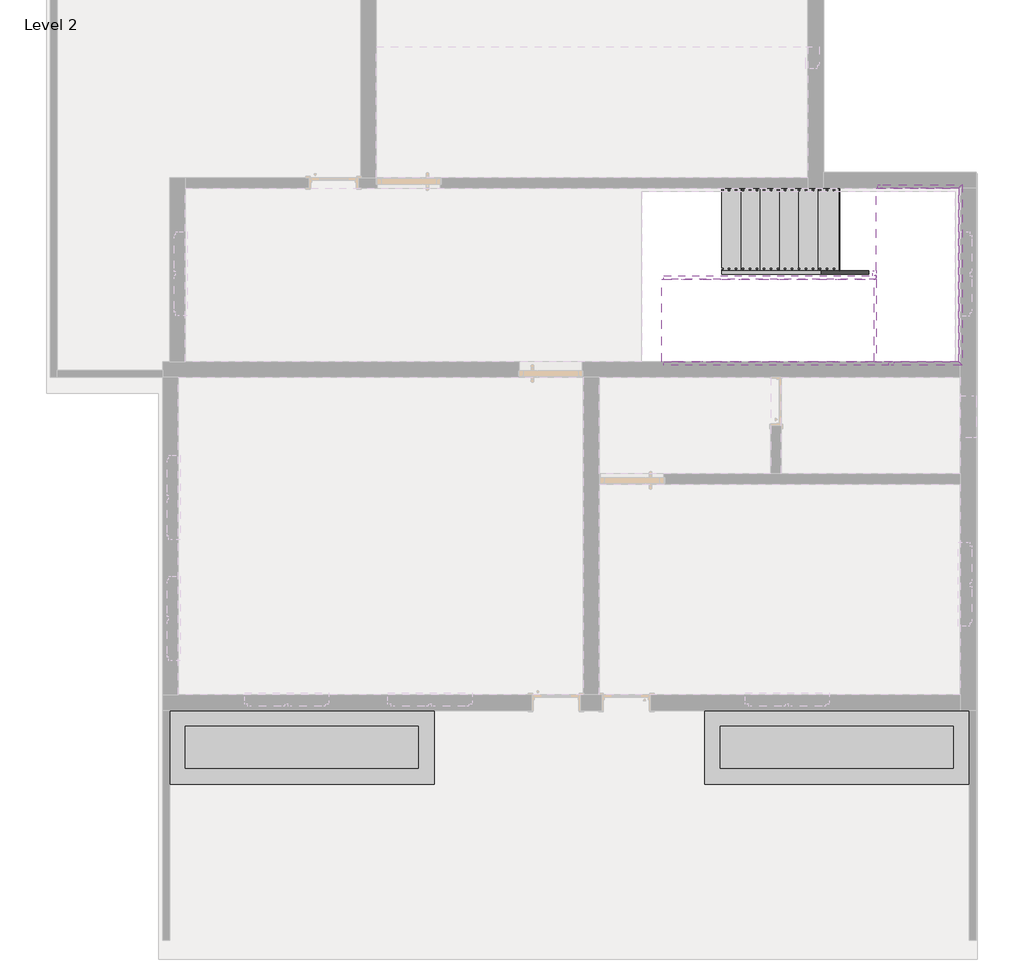
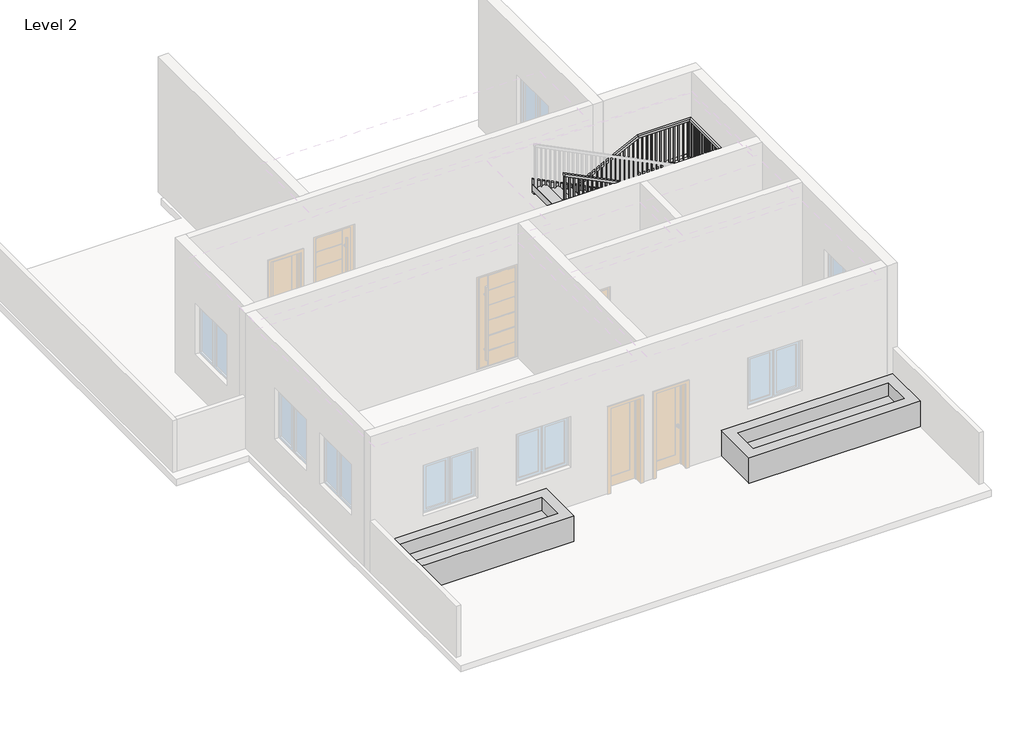
# One storey, part 3 of 3: 8 members, 2 stair flights, 1 proxy, 1 railing, 1 slab.
"""IFC4 building model written with IfcOpenShell, lengths in millimetres."""

from ifc_helpers import new_model, si_unit, frame, origin, place, context, project, spatial, polyline, outline, extrude, faceted_brep, transform, mapped, element, save
from components import generic_models_2_generic_models_2_98d2fe3e, non_monolithic_landing_0d67d91a, stair_flight_e1fa31a4, stair_flight_7751b166

model = new_model("IFC4")

# Units and contexts
model_context = context("Model", 3, world=origin())
ifc_project = project(units=[si_unit("LENGTHUNIT", "METRE", prefix="MILLI")], contexts=[model_context])

# Site, building, storey
site = spatial("IfcSite", under=ifc_project)
building = spatial("IfcBuilding", under=site)
storey = spatial("IfcBuildingStorey", under=building, Name="Level 2", Elevation=3200.4)

# Proxy
placement = place(None, origin())
generic_models_2_generic_models_2_shape = generic_models_2_generic_models_2_98d2fe3e(model_context)
element("IfcBuildingElementProxy", 1, Name="Generic Models 2 : Generic Models 2", ObjectType="Generic Models 2 : Generic Models 2", at=placement, inside=storey, context=model_context, shape_type="MappedRepresentation", body=[
    mapped(generic_models_2_generic_models_2_shape, transform((0.0, 0.0, 0.0), x_axis=(1.0, 0.0, 0.0), y_axis=(0.0, 1.0, 0.0), z_axis=(0.0, 0.0, 1.0))),
])

# Members
element("IfcMember", 2, ObjectType="Stringer - 2\" Width", at=placement, inside=storey, context=model_context, shape_type="SweptSolid", body=[
    extrude(outline(polyline([(3681.6520721, -12169.2183666), (3341.1442748, -12169.2183666), (4502.426087, -9837.43822), (4807.226087, -9909.1372097), (3681.6520721, -12169.2183666)])), frame((0.0, 3383.7503619, 0.0), z_axis=(0.0, 1.0, 0.0), x_axis=(0.0, 0.0, 1.0)), (0.0, 0.0, 1.0), 50.8),
])
element("IfcMember", 3, ObjectType="Stringer - 2\" Width", at=placement, inside=storey, context=model_context, shape_type="SweptSolid", body=[
    extrude(outline(polyline([(3681.6520721, -12169.2183666), (3341.1442748, -12169.2183666), (4429.0272787, -9984.8183666), (4769.535076, -9984.8183666), (3681.6520721, -12169.2183666)])), frame((0.0, 2139.1503619, 0.0), z_axis=(0.0, 1.0, 0.0), x_axis=(0.0, 0.0, 1.0)), (0.0, 0.0, 1.0), 50.8),
])
element("IfcMember", 4, ObjectType="Stringer - 2\" Width", at=placement, inside=storey, context=model_context, shape_type="SweptSolid", body=[
    extrude(outline(polyline([(4502.426087, -9751.1985133), (4807.226087, -9679.4995235), (6464.6085938, -13007.4183666), (6124.1007965, -13007.4183666), (4502.426087, -9751.1985133)])), frame((0.0, 818.3503619, 0.0), z_axis=(0.0, 1.0, 0.0), x_axis=(0.0, 0.0, 1.0)), (0.0, 0.0, 1.0), 50.8),
])
element("IfcMember", 5, ObjectType="Stringer - 2\" Width", at=placement, inside=storey, context=model_context, shape_type="SweptSolid", body=[
    extrude(outline(polyline([(4593.4747096, -9934.0183666), (4933.9825068, -9934.0183666), (6464.6085938, -13007.4183666), (6124.1007965, -13007.4183666), (4593.4747096, -9934.0183666)])), frame((0.0, 2062.9503619, 0.0), z_axis=(0.0, 1.0, 0.0), x_axis=(0.0, 0.0, 1.0)), (0.0, 0.0, 1.0), 50.8),
])
element("IfcMember", 6, ObjectType="Stringer - 2\" Width", at=placement, inside=storey, context=model_context, shape_type="Brep", body=[
    faceted_brep([(-9679.4995235, 869.1503619, 4807.226087), (-9679.4995235, 818.3503619, 4807.226087), (-8689.4183666, 818.3503619, 4807.226087), (-8740.2183666, 869.1503619, 4807.226087), (-9751.1985133, 869.1503619, 4502.426087), (-8740.2183666, 869.1503619, 4502.426087), (-9751.1985133, 818.3503619, 4502.426087), (-8689.4183666, 818.3503619, 4502.426087)], [[[0, 1, 2, 3]], [[4, 0, 3, 5]], [[6, 4, 5, 7]], [[1, 6, 7, 2]], [[1, 0, 4, 6]], [[2, 7, 5, 3]]]),
])
element("IfcMember", 7, ObjectType="Stringer - 2\" Width", at=placement, inside=storey, context=model_context, shape_type="SweptSolid", body=[
    extrude(outline(polyline([(-8689.4183666, 818.3503619), (-8740.2183666, 869.1503619), (-8740.2183666, 3383.7503619), (-8689.4183666, 3434.5503619), (-8689.4183666, 818.3503619)])), frame((0.0, 0.0, 4502.426087), z_axis=(0.0, 0.0, 1.0), x_axis=(1.0, 0.0, 0.0)), (0.0, 0.0, 1.0), 304.8),
])
element("IfcMember", 8, ObjectType="Stringer - 2\" Width", at=placement, inside=storey, context=model_context, shape_type="Brep", body=[
    faceted_brep([(-8740.2183666, 3383.7503619, 4807.226087), (-8689.4183666, 3434.5503619, 4807.226087), (-9909.1372097, 3434.5503619, 4807.226087), (-9909.1372097, 3383.7503619, 4807.226087), (-8740.2183666, 3383.7503619, 4502.426087), (-9837.43822, 3383.7503619, 4502.426087), (-8689.4183666, 3434.5503619, 4502.426087), (-9837.43822, 3434.5503619, 4502.426087)], [[[0, 1, 2, 3]], [[4, 0, 3, 5]], [[6, 4, 5, 7]], [[1, 6, 7, 2]], [[1, 0, 4, 6]], [[2, 7, 5, 3]]]),
])
element("IfcMember", 9, ObjectType="Stringer - 2\" Width", at=placement, inside=storey, context=model_context, shape_type="SweptSolid", body=[
    extrude(outline(polyline([(-9984.8183666, 2189.9503619), (-9934.0183666, 2189.9503619), (-9934.0183666, 2113.7503619), (-9984.8183666, 2113.7503619), (-9984.8183666, 2189.9503619)])), frame((0.0, 0.0, 4502.426087), z_axis=(0.0, 0.0, 1.0), x_axis=(1.0, 0.0, 0.0)), (0.0, 0.0, 1.0), 304.8),
])

# Railing
element("IfcRailing", 10, ObjectType="Handrail - Rectangular", at=placement, inside=storey, context=model_context, shape_type="SolidModel", body=[
    faceted_brep([(-12169.2183666, 3383.7503619, 4532.2434783), (-12169.2183666, 3383.7503619, 4475.4921787), (-12169.2183666, 3332.9503619, 4475.4921787), (-12169.2183666, 3332.9503619, 4532.2434783), (-9934.0183666, 3383.7503619, 5645.426087), (-9922.068535, 3383.7503619, 5594.626087), (-9922.068535, 3332.9503619, 5594.626087), (-9934.0183666, 3332.9503619, 5645.426087), (-8740.2183666, 3383.7503619, 5645.426087), (-8740.2183666, 3383.7503619, 5594.626087), (-8791.0183666, 3332.9503619, 5594.626087), (-8791.0183666, 3332.9503619, 5645.426087), (-8740.2183666, 869.1503619, 5645.426087), (-8740.2183666, 869.1503619, 5594.626087), (-8791.0183666, 919.9503619, 5594.626087), (-8791.0183666, 919.9503619, 5645.426087), (-9654.6183666, 869.1503619, 5645.426087), (-9666.5681983, 869.1503619, 5594.626087), (-9666.5681983, 919.9503619, 5594.626087), (-9654.6183666, 919.9503619, 5645.426087), (-9934.0183666, 869.1503619, 5784.573913), (-9956.6648951, 869.1503619, 5739.1011217), (-9956.6648951, 919.9503619, 5739.1011217), (-9934.0183666, 919.9503619, 5784.573913), (-13007.4183666, 869.1503619, 7315.2), (-13007.4183666, 919.9503619, 7315.2), (-13007.4183666, 919.9503619, 7258.4487005), (-13007.4183666, 869.1503619, 7258.4487005)], [[[0, 1, 2, 3]], [[1, 0, 4, 5]], [[2, 1, 5, 6]], [[3, 2, 6, 7]], [[0, 3, 7, 4]], [[5, 4, 8, 9]], [[6, 5, 9, 10]], [[7, 6, 10, 11]], [[4, 7, 11, 8]], [[9, 8, 12, 13]], [[10, 9, 13, 14]], [[11, 10, 14, 15]], [[8, 11, 15, 12]], [[13, 12, 16, 17]], [[14, 13, 17, 18]], [[15, 14, 18, 19]], [[12, 15, 19, 16]], [[17, 16, 20, 21]], [[18, 17, 21, 22]], [[19, 18, 22, 23]], [[16, 19, 23, 20]], [[24, 25, 26, 27]], [[21, 20, 24, 27]], [[22, 21, 27, 26]], [[23, 22, 26, 25]], [[20, 23, 25, 24]]]),
    extrude(outline(polyline([(7250.542574, -12991.5433666), (6261.6521739, -12991.5433666), (6261.6521739, -12972.4933666), (7241.0552222, -12972.4933666), (7250.542574, -12991.5433666)])), frame((0.0, 885.0253619, 0.0), z_axis=(0.0, 1.0, 0.0), x_axis=(0.0, 0.0, 1.0)), (0.0, 0.0, 1.0), 19.05),
    extrude(outline(polyline([(7199.9433645, -12889.9433666), (6261.6521739, -12889.9433666), (6261.6521739, -12870.8933666), (7190.4560127, -12870.8933666), (7199.9433645, -12889.9433666)])), frame((0.0, 885.0253619, 0.0), z_axis=(0.0, 1.0, 0.0), x_axis=(0.0, 0.0, 1.0)), (0.0, 0.0, 1.0), 19.05),
    extrude(outline(polyline([(7149.344155, -12788.3433666), (6261.6521739, -12788.3433666), (6261.6521739, -12769.2933666), (7139.8568032, -12769.2933666), (7149.344155, -12788.3433666)])), frame((0.0, 885.0253619, 0.0), z_axis=(0.0, 1.0, 0.0), x_axis=(0.0, 0.0, 1.0)), (0.0, 0.0, 1.0), 19.05),
    extrude(outline(polyline([(7098.7449455, -12686.7433666), (6122.5043478, -12686.7433666), (6122.5043478, -12667.6933666), (7089.2575937, -12667.6933666), (7098.7449455, -12686.7433666)])), frame((0.0, 885.0253619, 0.0), z_axis=(0.0, 1.0, 0.0), x_axis=(0.0, 0.0, 1.0)), (0.0, 0.0, 1.0), 19.05),
    extrude(outline(polyline([(7048.145736, -12585.1433666), (6122.5043478, -12585.1433666), (6122.5043478, -12566.0933666), (7038.6583842, -12566.0933666), (7048.145736, -12585.1433666)])), frame((0.0, 885.0253619, 0.0), z_axis=(0.0, 1.0, 0.0), x_axis=(0.0, 0.0, 1.0)), (0.0, 0.0, 1.0), 19.05),
    extrude(outline(polyline([(6997.5465265, -12483.5433666), (6122.5043478, -12483.5433666), (6122.5043478, -12464.4933666), (6988.0591748, -12464.4933666), (6997.5465265, -12483.5433666)])), frame((0.0, 885.0253619, 0.0), z_axis=(0.0, 1.0, 0.0), x_axis=(0.0, 0.0, 1.0)), (0.0, 0.0, 1.0), 19.05),
    extrude(outline(polyline([(6946.9473171, -12381.9433666), (5983.3565217, -12381.9433666), (5983.3565217, -12362.8933666), (6937.4599653, -12362.8933666), (6946.9473171, -12381.9433666)])), frame((0.0, 885.0253619, 0.0), z_axis=(0.0, 1.0, 0.0), x_axis=(0.0, 0.0, 1.0)), (0.0, 0.0, 1.0), 19.05),
    extrude(outline(polyline([(6896.3481076, -12280.3433666), (5983.3565217, -12280.3433666), (5983.3565217, -12261.2933666), (6886.8607558, -12261.2933666), (6896.3481076, -12280.3433666)])), frame((0.0, 885.0253619, 0.0), z_axis=(0.0, 1.0, 0.0), x_axis=(0.0, 0.0, 1.0)), (0.0, 0.0, 1.0), 19.05),
    extrude(outline(polyline([(6845.7488981, -12178.7433666), (5983.3565217, -12178.7433666), (5983.3565217, -12159.6933666), (6836.2615463, -12159.6933666), (6845.7488981, -12178.7433666)])), frame((0.0, 885.0253619, 0.0), z_axis=(0.0, 1.0, 0.0), x_axis=(0.0, 0.0, 1.0)), (0.0, 0.0, 1.0), 19.05),
    extrude(outline(polyline([(6795.1496886, -12077.1433666), (5844.2086957, -12077.1433666), (5844.2086957, -12058.0933666), (6785.6623368, -12058.0933666), (6795.1496886, -12077.1433666)])), frame((0.0, 885.0253619, 0.0), z_axis=(0.0, 1.0, 0.0), x_axis=(0.0, 0.0, 1.0)), (0.0, 0.0, 1.0), 19.05),
    extrude(outline(polyline([(6744.5504791, -11975.5433666), (5844.2086957, -11975.5433666), (5844.2086957, -11956.4933666), (6735.0631273, -11956.4933666), (6744.5504791, -11975.5433666)])), frame((0.0, 885.0253619, 0.0), z_axis=(0.0, 1.0, 0.0), x_axis=(0.0, 0.0, 1.0)), (0.0, 0.0, 1.0), 19.05),
    extrude(outline(polyline([(6693.9512696, -11873.9433666), (5705.0608696, -11873.9433666), (5705.0608696, -11854.8933666), (6684.4639178, -11854.8933666), (6693.9512696, -11873.9433666)])), frame((0.0, 885.0253619, 0.0), z_axis=(0.0, 1.0, 0.0), x_axis=(0.0, 0.0, 1.0)), (0.0, 0.0, 1.0), 19.05),
    extrude(outline(polyline([(6643.3520601, -11772.3433666), (5705.0608696, -11772.3433666), (5705.0608696, -11753.2933666), (6633.8647084, -11753.2933666), (6643.3520601, -11772.3433666)])), frame((0.0, 885.0253619, 0.0), z_axis=(0.0, 1.0, 0.0), x_axis=(0.0, 0.0, 1.0)), (0.0, 0.0, 1.0), 19.05),
    extrude(outline(polyline([(6592.7528507, -11670.7433666), (5705.0608696, -11670.7433666), (5705.0608696, -11651.6933666), (6583.2654989, -11651.6933666), (6592.7528507, -11670.7433666)])), frame((0.0, 885.0253619, 0.0), z_axis=(0.0, 1.0, 0.0), x_axis=(0.0, 0.0, 1.0)), (0.0, 0.0, 1.0), 19.05),
    extrude(outline(polyline([(6542.1536412, -11569.1433666), (5565.9130435, -11569.1433666), (5565.9130435, -11550.0933666), (6532.6662894, -11550.0933666), (6542.1536412, -11569.1433666)])), frame((0.0, 885.0253619, 0.0), z_axis=(0.0, 1.0, 0.0), x_axis=(0.0, 0.0, 1.0)), (0.0, 0.0, 1.0), 19.05),
    extrude(outline(polyline([(6491.5544317, -11467.5433666), (5565.9130435, -11467.5433666), (5565.9130435, -11448.4933666), (6482.0670799, -11448.4933666), (6491.5544317, -11467.5433666)])), frame((0.0, 885.0253619, 0.0), z_axis=(0.0, 1.0, 0.0), x_axis=(0.0, 0.0, 1.0)), (0.0, 0.0, 1.0), 19.05),
    extrude(outline(polyline([(6440.9552222, -11365.9433666), (5565.9130435, -11365.9433666), (5565.9130435, -11346.8933666), (6431.4678704, -11346.8933666), (6440.9552222, -11365.9433666)])), frame((0.0, 885.0253619, 0.0), z_axis=(0.0, 1.0, 0.0), x_axis=(0.0, 0.0, 1.0)), (0.0, 0.0, 1.0), 19.05),
    extrude(outline(polyline([(6390.3560127, -11264.3433666), (5426.7652174, -11264.3433666), (5426.7652174, -11245.2933666), (6380.8686609, -11245.2933666), (6390.3560127, -11264.3433666)])), frame((0.0, 885.0253619, 0.0), z_axis=(0.0, 1.0, 0.0), x_axis=(0.0, 0.0, 1.0)), (0.0, 0.0, 1.0), 19.05),
    extrude(outline(polyline([(6339.7568032, -11162.7433666), (5426.7652174, -11162.7433666), (5426.7652174, -11143.6933666), (6330.2694514, -11143.6933666), (6339.7568032, -11162.7433666)])), frame((0.0, 885.0253619, 0.0), z_axis=(0.0, 1.0, 0.0), x_axis=(0.0, 0.0, 1.0)), (0.0, 0.0, 1.0), 19.05),
    extrude(outline(polyline([(6289.1575937, -11061.1433666), (5426.7652174, -11061.1433666), (5426.7652174, -11042.0933666), (6279.670242, -11042.0933666), (6289.1575937, -11061.1433666)])), frame((0.0, 885.0253619, 0.0), z_axis=(0.0, 1.0, 0.0), x_axis=(0.0, 0.0, 1.0)), (0.0, 0.0, 1.0), 19.05),
    extrude(outline(polyline([(6238.5583842, -10959.5433666), (5287.6173913, -10959.5433666), (5287.6173913, -10940.4933666), (6229.0710325, -10940.4933666), (6238.5583842, -10959.5433666)])), frame((0.0, 885.0253619, 0.0), z_axis=(0.0, 1.0, 0.0), x_axis=(0.0, 0.0, 1.0)), (0.0, 0.0, 1.0), 19.05),
    extrude(outline(polyline([(6187.9591748, -10857.9433666), (5287.6173913, -10857.9433666), (5287.6173913, -10838.8933666), (6178.471823, -10838.8933666), (6187.9591748, -10857.9433666)])), frame((0.0, 885.0253619, 0.0), z_axis=(0.0, 1.0, 0.0), x_axis=(0.0, 0.0, 1.0)), (0.0, 0.0, 1.0), 19.05),
    extrude(outline(polyline([(6137.3599653, -10756.3433666), (5148.4695652, -10756.3433666), (5148.4695652, -10737.2933666), (6127.8726135, -10737.2933666), (6137.3599653, -10756.3433666)])), frame((0.0, 885.0253619, 0.0), z_axis=(0.0, 1.0, 0.0), x_axis=(0.0, 0.0, 1.0)), (0.0, 0.0, 1.0), 19.05),
    extrude(outline(polyline([(6086.7607558, -10654.7433666), (5148.4695652, -10654.7433666), (5148.4695652, -10635.6933666), (6077.273404, -10635.6933666), (6086.7607558, -10654.7433666)])), frame((0.0, 885.0253619, 0.0), z_axis=(0.0, 1.0, 0.0), x_axis=(0.0, 0.0, 1.0)), (0.0, 0.0, 1.0), 19.05),
    extrude(outline(polyline([(6036.1615463, -10553.1433666), (5148.4695652, -10553.1433666), (5148.4695652, -10534.0933666), (6026.6741945, -10534.0933666), (6036.1615463, -10553.1433666)])), frame((0.0, 885.0253619, 0.0), z_axis=(0.0, 1.0, 0.0), x_axis=(0.0, 0.0, 1.0)), (0.0, 0.0, 1.0), 19.05),
    extrude(outline(polyline([(5985.5623368, -10451.5433666), (5009.3217391, -10451.5433666), (5009.3217391, -10432.4933666), (5976.074985, -10432.4933666), (5985.5623368, -10451.5433666)])), frame((0.0, 885.0253619, 0.0), z_axis=(0.0, 1.0, 0.0), x_axis=(0.0, 0.0, 1.0)), (0.0, 0.0, 1.0), 19.05),
    extrude(outline(polyline([(5934.9631273, -10349.9433666), (5009.3217391, -10349.9433666), (5009.3217391, -10330.8933666), (5925.4757756, -10330.8933666), (5934.9631273, -10349.9433666)])), frame((0.0, 885.0253619, 0.0), z_axis=(0.0, 1.0, 0.0), x_axis=(0.0, 0.0, 1.0)), (0.0, 0.0, 1.0), 19.05),
    extrude(outline(polyline([(5884.3639178, -10248.3433666), (5009.3217391, -10248.3433666), (5009.3217391, -10229.2933666), (5874.8765661, -10229.2933666), (5884.3639178, -10248.3433666)])), frame((0.0, 885.0253619, 0.0), z_axis=(0.0, 1.0, 0.0), x_axis=(0.0, 0.0, 1.0)), (0.0, 0.0, 1.0), 19.05),
    extrude(outline(polyline([(5833.7647084, -10146.7433666), (4870.173913, -10146.7433666), (4870.173913, -10127.6933666), (5824.2773566, -10127.6933666), (5833.7647084, -10146.7433666)])), frame((0.0, 885.0253619, 0.0), z_axis=(0.0, 1.0, 0.0), x_axis=(0.0, 0.0, 1.0)), (0.0, 0.0, 1.0), 19.05),
    extrude(outline(polyline([(5783.1654989, -10045.1433666), (4870.173913, -10045.1433666), (4870.173913, -10026.0933666), (5773.6781471, -10026.0933666), (5783.1654989, -10045.1433666)])), frame((0.0, 885.0253619, 0.0), z_axis=(0.0, 1.0, 0.0), x_axis=(0.0, 0.0, 1.0)), (0.0, 0.0, 1.0), 19.05),
    extrude(outline(polyline([(5707.2666846, -9892.7433666), (4731.026087, -9892.7433666), (4731.026087, -9873.6933666), (5697.7793329, -9873.6933666), (5707.2666846, -9892.7433666)])), frame((0.0, 885.0253619, 0.0), z_axis=(0.0, 1.0, 0.0), x_axis=(0.0, 0.0, 1.0)), (0.0, 0.0, 1.0), 19.05),
    extrude(outline(polyline([(5656.6674752, -9791.1433666), (4731.026087, -9791.1433666), (4731.026087, -9772.0933666), (5647.1801234, -9772.0933666), (5656.6674752, -9791.1433666)])), frame((0.0, 885.0253619, 0.0), z_axis=(0.0, 1.0, 0.0), x_axis=(0.0, 0.0, 1.0)), (0.0, 0.0, 1.0), 19.05),
    extrude(outline(polyline([(5606.0682657, -9689.5433666), (4731.026087, -9689.5433666), (4731.026087, -9670.4933666), (5596.5809139, -9670.4933666), (5606.0682657, -9689.5433666)])), frame((0.0, 885.0253619, 0.0), z_axis=(0.0, 1.0, 0.0), x_axis=(0.0, 0.0, 1.0)), (0.0, 0.0, 1.0), 19.05),
    extrude(outline(polyline([(-9568.8933666, 885.0253619), (-9587.9433666, 885.0253619), (-9587.9433666, 904.0753619), (-9568.8933666, 904.0753619), (-9568.8933666, 885.0253619)])), frame((0.0, 0.0, 4731.026087), z_axis=(0.0, 0.0, 1.0), x_axis=(1.0, 0.0, 0.0)), (0.0, 0.0, 1.0), 863.6),
    extrude(outline(polyline([(-9467.2933666, 885.0253619), (-9486.3433666, 885.0253619), (-9486.3433666, 904.0753619), (-9467.2933666, 904.0753619), (-9467.2933666, 885.0253619)])), frame((0.0, 0.0, 4731.026087), z_axis=(0.0, 0.0, 1.0), x_axis=(1.0, 0.0, 0.0)), (0.0, 0.0, 1.0), 863.6),
    extrude(outline(polyline([(-9365.6933666, 885.0253619), (-9384.7433666, 885.0253619), (-9384.7433666, 904.0753619), (-9365.6933666, 904.0753619), (-9365.6933666, 885.0253619)])), frame((0.0, 0.0, 4731.026087), z_axis=(0.0, 0.0, 1.0), x_axis=(1.0, 0.0, 0.0)), (0.0, 0.0, 1.0), 863.6),
    extrude(outline(polyline([(-9264.0933666, 885.0253619), (-9283.1433666, 885.0253619), (-9283.1433666, 904.0753619), (-9264.0933666, 904.0753619), (-9264.0933666, 885.0253619)])), frame((0.0, 0.0, 4731.026087), z_axis=(0.0, 0.0, 1.0), x_axis=(1.0, 0.0, 0.0)), (0.0, 0.0, 1.0), 863.6),
    extrude(outline(polyline([(-9162.4933666, 885.0253619), (-9181.5433666, 885.0253619), (-9181.5433666, 904.0753619), (-9162.4933666, 904.0753619), (-9162.4933666, 885.0253619)])), frame((0.0, 0.0, 4731.026087), z_axis=(0.0, 0.0, 1.0), x_axis=(1.0, 0.0, 0.0)), (0.0, 0.0, 1.0), 863.6),
    extrude(outline(polyline([(-9060.8933666, 885.0253619), (-9079.9433666, 885.0253619), (-9079.9433666, 904.0753619), (-9060.8933666, 904.0753619), (-9060.8933666, 885.0253619)])), frame((0.0, 0.0, 4731.026087), z_axis=(0.0, 0.0, 1.0), x_axis=(1.0, 0.0, 0.0)), (0.0, 0.0, 1.0), 863.6),
    extrude(outline(polyline([(-8959.2933666, 885.0253619), (-8978.3433666, 885.0253619), (-8978.3433666, 904.0753619), (-8959.2933666, 904.0753619), (-8959.2933666, 885.0253619)])), frame((0.0, 0.0, 4731.026087), z_axis=(0.0, 0.0, 1.0), x_axis=(1.0, 0.0, 0.0)), (0.0, 0.0, 1.0), 863.6),
    extrude(outline(polyline([(-8857.6933666, 885.0253619), (-8876.7433666, 885.0253619), (-8876.7433666, 904.0753619), (-8857.6933666, 904.0753619), (-8857.6933666, 885.0253619)])), frame((0.0, 0.0, 4731.026087), z_axis=(0.0, 0.0, 1.0), x_axis=(1.0, 0.0, 0.0)), (0.0, 0.0, 1.0), 863.6),
    extrude(outline(polyline([(-8756.0933666, 929.4753619), (-8756.0933666, 910.4253619), (-8775.1433666, 910.4253619), (-8775.1433666, 929.4753619), (-8756.0933666, 929.4753619)])), frame((0.0, 0.0, 4731.026087), z_axis=(0.0, 0.0, 1.0), x_axis=(1.0, 0.0, 0.0)), (0.0, 0.0, 1.0), 863.6),
    extrude(outline(polyline([(-8756.0933666, 1031.0753619), (-8756.0933666, 1012.0253619), (-8775.1433666, 1012.0253619), (-8775.1433666, 1031.0753619), (-8756.0933666, 1031.0753619)])), frame((0.0, 0.0, 4731.026087), z_axis=(0.0, 0.0, 1.0), x_axis=(1.0, 0.0, 0.0)), (0.0, 0.0, 1.0), 863.6),
    extrude(outline(polyline([(-8756.0933666, 1132.6753619), (-8756.0933666, 1113.6253619), (-8775.1433666, 1113.6253619), (-8775.1433666, 1132.6753619), (-8756.0933666, 1132.6753619)])), frame((0.0, 0.0, 4731.026087), z_axis=(0.0, 0.0, 1.0), x_axis=(1.0, 0.0, 0.0)), (0.0, 0.0, 1.0), 863.6),
    extrude(outline(polyline([(-8756.0933666, 1234.2753619), (-8756.0933666, 1215.2253619), (-8775.1433666, 1215.2253619), (-8775.1433666, 1234.2753619), (-8756.0933666, 1234.2753619)])), frame((0.0, 0.0, 4731.026087), z_axis=(0.0, 0.0, 1.0), x_axis=(1.0, 0.0, 0.0)), (0.0, 0.0, 1.0), 863.6),
    extrude(outline(polyline([(-8756.0933666, 1335.8753619), (-8756.0933666, 1316.8253619), (-8775.1433666, 1316.8253619), (-8775.1433666, 1335.8753619), (-8756.0933666, 1335.8753619)])), frame((0.0, 0.0, 4731.026087), z_axis=(0.0, 0.0, 1.0), x_axis=(1.0, 0.0, 0.0)), (0.0, 0.0, 1.0), 863.6),
    extrude(outline(polyline([(-8756.0933666, 1437.4753619), (-8756.0933666, 1418.4253619), (-8775.1433666, 1418.4253619), (-8775.1433666, 1437.4753619), (-8756.0933666, 1437.4753619)])), frame((0.0, 0.0, 4731.026087), z_axis=(0.0, 0.0, 1.0), x_axis=(1.0, 0.0, 0.0)), (0.0, 0.0, 1.0), 863.6),
    extrude(outline(polyline([(-8756.0933666, 1539.0753619), (-8756.0933666, 1520.0253619), (-8775.1433666, 1520.0253619), (-8775.1433666, 1539.0753619), (-8756.0933666, 1539.0753619)])), frame((0.0, 0.0, 4731.026087), z_axis=(0.0, 0.0, 1.0), x_axis=(1.0, 0.0, 0.0)), (0.0, 0.0, 1.0), 863.6),
    extrude(outline(polyline([(-8756.0933666, 1640.6753619), (-8756.0933666, 1621.6253619), (-8775.1433666, 1621.6253619), (-8775.1433666, 1640.6753619), (-8756.0933666, 1640.6753619)])), frame((0.0, 0.0, 4731.026087), z_axis=(0.0, 0.0, 1.0), x_axis=(1.0, 0.0, 0.0)), (0.0, 0.0, 1.0), 863.6),
    extrude(outline(polyline([(-8756.0933666, 1742.2753619), (-8756.0933666, 1723.2253619), (-8775.1433666, 1723.2253619), (-8775.1433666, 1742.2753619), (-8756.0933666, 1742.2753619)])), frame((0.0, 0.0, 4731.026087), z_axis=(0.0, 0.0, 1.0), x_axis=(1.0, 0.0, 0.0)), (0.0, 0.0, 1.0), 863.6),
    extrude(outline(polyline([(-8756.0933666, 1843.8753619), (-8756.0933666, 1824.8253619), (-8775.1433666, 1824.8253619), (-8775.1433666, 1843.8753619), (-8756.0933666, 1843.8753619)])), frame((0.0, 0.0, 4731.026087), z_axis=(0.0, 0.0, 1.0), x_axis=(1.0, 0.0, 0.0)), (0.0, 0.0, 1.0), 863.6),
    extrude(outline(polyline([(-8756.0933666, 1945.4753619), (-8756.0933666, 1926.4253619), (-8775.1433666, 1926.4253619), (-8775.1433666, 1945.4753619), (-8756.0933666, 1945.4753619)])), frame((0.0, 0.0, 4731.026087), z_axis=(0.0, 0.0, 1.0), x_axis=(1.0, 0.0, 0.0)), (0.0, 0.0, 1.0), 863.6),
    extrude(outline(polyline([(-8756.0933666, 2047.0753619), (-8756.0933666, 2028.0253619), (-8775.1433666, 2028.0253619), (-8775.1433666, 2047.0753619), (-8756.0933666, 2047.0753619)])), frame((0.0, 0.0, 4731.026087), z_axis=(0.0, 0.0, 1.0), x_axis=(1.0, 0.0, 0.0)), (0.0, 0.0, 1.0), 863.6),
    extrude(outline(polyline([(-8756.0933666, 2148.6753619), (-8756.0933666, 2129.6253619), (-8775.1433666, 2129.6253619), (-8775.1433666, 2148.6753619), (-8756.0933666, 2148.6753619)])), frame((0.0, 0.0, 4731.026087), z_axis=(0.0, 0.0, 1.0), x_axis=(1.0, 0.0, 0.0)), (0.0, 0.0, 1.0), 863.6),
    extrude(outline(polyline([(-8756.0933666, 2250.2753619), (-8756.0933666, 2231.2253619), (-8775.1433666, 2231.2253619), (-8775.1433666, 2250.2753619), (-8756.0933666, 2250.2753619)])), frame((0.0, 0.0, 4731.026087), z_axis=(0.0, 0.0, 1.0), x_axis=(1.0, 0.0, 0.0)), (0.0, 0.0, 1.0), 863.6),
    extrude(outline(polyline([(-8756.0933666, 2351.8753619), (-8756.0933666, 2332.8253619), (-8775.1433666, 2332.8253619), (-8775.1433666, 2351.8753619), (-8756.0933666, 2351.8753619)])), frame((0.0, 0.0, 4731.026087), z_axis=(0.0, 0.0, 1.0), x_axis=(1.0, 0.0, 0.0)), (0.0, 0.0, 1.0), 863.6),
    extrude(outline(polyline([(-8756.0933666, 2453.4753619), (-8756.0933666, 2434.4253619), (-8775.1433666, 2434.4253619), (-8775.1433666, 2453.4753619), (-8756.0933666, 2453.4753619)])), frame((0.0, 0.0, 4731.026087), z_axis=(0.0, 0.0, 1.0), x_axis=(1.0, 0.0, 0.0)), (0.0, 0.0, 1.0), 863.6),
    extrude(outline(polyline([(-8756.0933666, 2555.0753619), (-8756.0933666, 2536.0253619), (-8775.1433666, 2536.0253619), (-8775.1433666, 2555.0753619), (-8756.0933666, 2555.0753619)])), frame((0.0, 0.0, 4731.026087), z_axis=(0.0, 0.0, 1.0), x_axis=(1.0, 0.0, 0.0)), (0.0, 0.0, 1.0), 863.6),
    extrude(outline(polyline([(-8756.0933666, 2656.6753619), (-8756.0933666, 2637.6253619), (-8775.1433666, 2637.6253619), (-8775.1433666, 2656.6753619), (-8756.0933666, 2656.6753619)])), frame((0.0, 0.0, 4731.026087), z_axis=(0.0, 0.0, 1.0), x_axis=(1.0, 0.0, 0.0)), (0.0, 0.0, 1.0), 863.6),
    extrude(outline(polyline([(-8756.0933666, 2758.2753619), (-8756.0933666, 2739.2253619), (-8775.1433666, 2739.2253619), (-8775.1433666, 2758.2753619), (-8756.0933666, 2758.2753619)])), frame((0.0, 0.0, 4731.026087), z_axis=(0.0, 0.0, 1.0), x_axis=(1.0, 0.0, 0.0)), (0.0, 0.0, 1.0), 863.6),
    extrude(outline(polyline([(-8756.0933666, 2859.8753619), (-8756.0933666, 2840.8253619), (-8775.1433666, 2840.8253619), (-8775.1433666, 2859.8753619), (-8756.0933666, 2859.8753619)])), frame((0.0, 0.0, 4731.026087), z_axis=(0.0, 0.0, 1.0), x_axis=(1.0, 0.0, 0.0)), (0.0, 0.0, 1.0), 863.6),
    extrude(outline(polyline([(-8756.0933666, 2961.4753619), (-8756.0933666, 2942.4253619), (-8775.1433666, 2942.4253619), (-8775.1433666, 2961.4753619), (-8756.0933666, 2961.4753619)])), frame((0.0, 0.0, 4731.026087), z_axis=(0.0, 0.0, 1.0), x_axis=(1.0, 0.0, 0.0)), (0.0, 0.0, 1.0), 863.6),
    extrude(outline(polyline([(-8756.0933666, 3063.0753619), (-8756.0933666, 3044.0253619), (-8775.1433666, 3044.0253619), (-8775.1433666, 3063.0753619), (-8756.0933666, 3063.0753619)])), frame((0.0, 0.0, 4731.026087), z_axis=(0.0, 0.0, 1.0), x_axis=(1.0, 0.0, 0.0)), (0.0, 0.0, 1.0), 863.6),
    extrude(outline(polyline([(-8756.0933666, 3164.6753619), (-8756.0933666, 3145.6253619), (-8775.1433666, 3145.6253619), (-8775.1433666, 3164.6753619), (-8756.0933666, 3164.6753619)])), frame((0.0, 0.0, 4731.026087), z_axis=(0.0, 0.0, 1.0), x_axis=(1.0, 0.0, 0.0)), (0.0, 0.0, 1.0), 863.6),
    extrude(outline(polyline([(-8756.0933666, 3266.2753619), (-8756.0933666, 3247.2253619), (-8775.1433666, 3247.2253619), (-8775.1433666, 3266.2753619), (-8756.0933666, 3266.2753619)])), frame((0.0, 0.0, 4731.026087), z_axis=(0.0, 0.0, 1.0), x_axis=(1.0, 0.0, 0.0)), (0.0, 0.0, 1.0), 863.6),
    extrude(outline(polyline([(-8825.9433666, 3367.8753619), (-8806.8933666, 3367.8753619), (-8806.8933666, 3348.8253619), (-8825.9433666, 3348.8253619), (-8825.9433666, 3367.8753619)])), frame((0.0, 0.0, 4731.026087), z_axis=(0.0, 0.0, 1.0), x_axis=(1.0, 0.0, 0.0)), (0.0, 0.0, 1.0), 863.6),
    extrude(outline(polyline([(-8927.5433666, 3367.8753619), (-8908.4933666, 3367.8753619), (-8908.4933666, 3348.8253619), (-8927.5433666, 3348.8253619), (-8927.5433666, 3367.8753619)])), frame((0.0, 0.0, 4731.026087), z_axis=(0.0, 0.0, 1.0), x_axis=(1.0, 0.0, 0.0)), (0.0, 0.0, 1.0), 863.6),
    extrude(outline(polyline([(-9029.1433666, 3367.8753619), (-9010.0933666, 3367.8753619), (-9010.0933666, 3348.8253619), (-9029.1433666, 3348.8253619), (-9029.1433666, 3367.8753619)])), frame((0.0, 0.0, 4731.026087), z_axis=(0.0, 0.0, 1.0), x_axis=(1.0, 0.0, 0.0)), (0.0, 0.0, 1.0), 863.6),
    extrude(outline(polyline([(-9130.7433666, 3367.8753619), (-9111.6933666, 3367.8753619), (-9111.6933666, 3348.8253619), (-9130.7433666, 3348.8253619), (-9130.7433666, 3367.8753619)])), frame((0.0, 0.0, 4731.026087), z_axis=(0.0, 0.0, 1.0), x_axis=(1.0, 0.0, 0.0)), (0.0, 0.0, 1.0), 863.6),
    extrude(outline(polyline([(-9232.3433666, 3367.8753619), (-9213.2933666, 3367.8753619), (-9213.2933666, 3348.8253619), (-9232.3433666, 3348.8253619), (-9232.3433666, 3367.8753619)])), frame((0.0, 0.0, 4731.026087), z_axis=(0.0, 0.0, 1.0), x_axis=(1.0, 0.0, 0.0)), (0.0, 0.0, 1.0), 863.6),
    extrude(outline(polyline([(-9333.9433666, 3367.8753619), (-9314.8933666, 3367.8753619), (-9314.8933666, 3348.8253619), (-9333.9433666, 3348.8253619), (-9333.9433666, 3367.8753619)])), frame((0.0, 0.0, 4731.026087), z_axis=(0.0, 0.0, 1.0), x_axis=(1.0, 0.0, 0.0)), (0.0, 0.0, 1.0), 863.6),
    extrude(outline(polyline([(-9435.5433666, 3367.8753619), (-9416.4933666, 3367.8753619), (-9416.4933666, 3348.8253619), (-9435.5433666, 3348.8253619), (-9435.5433666, 3367.8753619)])), frame((0.0, 0.0, 4731.026087), z_axis=(0.0, 0.0, 1.0), x_axis=(1.0, 0.0, 0.0)), (0.0, 0.0, 1.0), 863.6),
    extrude(outline(polyline([(-9537.1433666, 3367.8753619), (-9518.0933666, 3367.8753619), (-9518.0933666, 3348.8253619), (-9537.1433666, 3348.8253619), (-9537.1433666, 3367.8753619)])), frame((0.0, 0.0, 4731.026087), z_axis=(0.0, 0.0, 1.0), x_axis=(1.0, 0.0, 0.0)), (0.0, 0.0, 1.0), 863.6),
    extrude(outline(polyline([(-9638.7433666, 3367.8753619), (-9619.6933666, 3367.8753619), (-9619.6933666, 3348.8253619), (-9638.7433666, 3348.8253619), (-9638.7433666, 3367.8753619)])), frame((0.0, 0.0, 4731.026087), z_axis=(0.0, 0.0, 1.0), x_axis=(1.0, 0.0, 0.0)), (0.0, 0.0, 1.0), 863.6),
    extrude(outline(polyline([(-9740.3433666, 3367.8753619), (-9721.2933666, 3367.8753619), (-9721.2933666, 3348.8253619), (-9740.3433666, 3348.8253619), (-9740.3433666, 3367.8753619)])), frame((0.0, 0.0, 4731.026087), z_axis=(0.0, 0.0, 1.0), x_axis=(1.0, 0.0, 0.0)), (0.0, 0.0, 1.0), 863.6),
    extrude(outline(polyline([(-9841.9433666, 3367.8753619), (-9822.8933666, 3367.8753619), (-9822.8933666, 3348.8253619), (-9841.9433666, 3348.8253619), (-9841.9433666, 3367.8753619)])), frame((0.0, 0.0, 4731.026087), z_axis=(0.0, 0.0, 1.0), x_axis=(1.0, 0.0, 0.0)), (0.0, 0.0, 1.0), 863.6),
    extrude(outline(polyline([(5533.331902, -10045.1433666), (4591.8782609, -10045.1433666), (4591.8782609, -10026.0933666), (5542.8192538, -10026.0933666), (5533.331902, -10045.1433666)])), frame((0.0, 3348.8253619, 0.0), z_axis=(0.0, 1.0, 0.0), x_axis=(0.0, 0.0, 1.0)), (0.0, 0.0, 1.0), 19.05),
    extrude(outline(polyline([(5482.7326925, -10146.7433666), (4591.8782609, -10146.7433666), (4591.8782609, -10127.6933666), (5492.2200443, -10127.6933666), (5482.7326925, -10146.7433666)])), frame((0.0, 3348.8253619, 0.0), z_axis=(0.0, 1.0, 0.0), x_axis=(0.0, 0.0, 1.0)), (0.0, 0.0, 1.0), 19.05),
    extrude(outline(polyline([(5432.1334831, -10248.3433666), (4452.7304348, -10248.3433666), (4452.7304348, -10229.2933666), (5441.6208348, -10229.2933666), (5432.1334831, -10248.3433666)])), frame((0.0, 3348.8253619, 0.0), z_axis=(0.0, 1.0, 0.0), x_axis=(0.0, 0.0, 1.0)), (0.0, 0.0, 1.0), 19.05),
    extrude(outline(polyline([(5381.5342736, -10349.9433666), (4452.7304348, -10349.9433666), (4452.7304348, -10330.8933666), (5391.0216254, -10330.8933666), (5381.5342736, -10349.9433666)])), frame((0.0, 3348.8253619, 0.0), z_axis=(0.0, 1.0, 0.0), x_axis=(0.0, 0.0, 1.0)), (0.0, 0.0, 1.0), 19.05),
    extrude(outline(polyline([(5330.9350641, -10451.5433666), (4452.7304348, -10451.5433666), (4452.7304348, -10432.4933666), (5340.4224159, -10432.4933666), (5330.9350641, -10451.5433666)])), frame((0.0, 3348.8253619, 0.0), z_axis=(0.0, 1.0, 0.0), x_axis=(0.0, 0.0, 1.0)), (0.0, 0.0, 1.0), 19.05),
    extrude(outline(polyline([(5280.3358546, -10553.1433666), (4313.5826087, -10553.1433666), (4313.5826087, -10534.0933666), (5289.8232064, -10534.0933666), (5280.3358546, -10553.1433666)])), frame((0.0, 3348.8253619, 0.0), z_axis=(0.0, 1.0, 0.0), x_axis=(0.0, 0.0, 1.0)), (0.0, 0.0, 1.0), 19.05),
    extrude(outline(polyline([(5229.7366451, -10654.7433666), (4313.5826087, -10654.7433666), (4313.5826087, -10635.6933666), (5239.2239969, -10635.6933666), (5229.7366451, -10654.7433666)])), frame((0.0, 3348.8253619, 0.0), z_axis=(0.0, 1.0, 0.0), x_axis=(0.0, 0.0, 1.0)), (0.0, 0.0, 1.0), 19.05),
    extrude(outline(polyline([(5179.1374356, -10756.3433666), (4313.5826087, -10756.3433666), (4313.5826087, -10737.2933666), (5188.6247874, -10737.2933666), (5179.1374356, -10756.3433666)])), frame((0.0, 3348.8253619, 0.0), z_axis=(0.0, 1.0, 0.0), x_axis=(0.0, 0.0, 1.0)), (0.0, 0.0, 1.0), 19.05),
    extrude(outline(polyline([(5128.5382261, -10857.9433666), (4174.4347826, -10857.9433666), (4174.4347826, -10838.8933666), (5138.0255779, -10838.8933666), (5128.5382261, -10857.9433666)])), frame((0.0, 3348.8253619, 0.0), z_axis=(0.0, 1.0, 0.0), x_axis=(0.0, 0.0, 1.0)), (0.0, 0.0, 1.0), 19.05),
    extrude(outline(polyline([(5077.9390167, -10959.5433666), (4174.4347826, -10959.5433666), (4174.4347826, -10940.4933666), (5087.4263684, -10940.4933666), (5077.9390167, -10959.5433666)])), frame((0.0, 3348.8253619, 0.0), z_axis=(0.0, 1.0, 0.0), x_axis=(0.0, 0.0, 1.0)), (0.0, 0.0, 1.0), 19.05),
    extrude(outline(polyline([(5027.3398072, -11061.1433666), (4174.4347826, -11061.1433666), (4174.4347826, -11042.0933666), (5036.827159, -11042.0933666), (5027.3398072, -11061.1433666)])), frame((0.0, 3348.8253619, 0.0), z_axis=(0.0, 1.0, 0.0), x_axis=(0.0, 0.0, 1.0)), (0.0, 0.0, 1.0), 19.05),
    extrude(outline(polyline([(4976.7405977, -11162.7433666), (4035.2869565, -11162.7433666), (4035.2869565, -11143.6933666), (4986.2279495, -11143.6933666), (4976.7405977, -11162.7433666)])), frame((0.0, 3348.8253619, 0.0), z_axis=(0.0, 1.0, 0.0), x_axis=(0.0, 0.0, 1.0)), (0.0, 0.0, 1.0), 19.05),
    extrude(outline(polyline([(4926.1413882, -11264.3433666), (4035.2869565, -11264.3433666), (4035.2869565, -11245.2933666), (4935.62874, -11245.2933666), (4926.1413882, -11264.3433666)])), frame((0.0, 3348.8253619, 0.0), z_axis=(0.0, 1.0, 0.0), x_axis=(0.0, 0.0, 1.0)), (0.0, 0.0, 1.0), 19.05),
    extrude(outline(polyline([(4875.5421787, -11365.9433666), (3896.1391304, -11365.9433666), (3896.1391304, -11346.8933666), (4885.0295305, -11346.8933666), (4875.5421787, -11365.9433666)])), frame((0.0, 3348.8253619, 0.0), z_axis=(0.0, 1.0, 0.0), x_axis=(0.0, 0.0, 1.0)), (0.0, 0.0, 1.0), 19.05),
    extrude(outline(polyline([(4824.9429692, -11467.5433666), (3896.1391304, -11467.5433666), (3896.1391304, -11448.4933666), (4834.430321, -11448.4933666), (4824.9429692, -11467.5433666)])), frame((0.0, 3348.8253619, 0.0), z_axis=(0.0, 1.0, 0.0), x_axis=(0.0, 0.0, 1.0)), (0.0, 0.0, 1.0), 19.05),
    extrude(outline(polyline([(4774.3437597, -11569.1433666), (3896.1391304, -11569.1433666), (3896.1391304, -11550.0933666), (4783.8311115, -11550.0933666), (4774.3437597, -11569.1433666)])), frame((0.0, 3348.8253619, 0.0), z_axis=(0.0, 1.0, 0.0), x_axis=(0.0, 0.0, 1.0)), (0.0, 0.0, 1.0), 19.05),
    extrude(outline(polyline([(4723.7445503, -11670.7433666), (3756.9913043, -11670.7433666), (3756.9913043, -11651.6933666), (4733.231902, -11651.6933666), (4723.7445503, -11670.7433666)])), frame((0.0, 3348.8253619, 0.0), z_axis=(0.0, 1.0, 0.0), x_axis=(0.0, 0.0, 1.0)), (0.0, 0.0, 1.0), 19.05),
    extrude(outline(polyline([(4673.1453408, -11772.3433666), (3756.9913043, -11772.3433666), (3756.9913043, -11753.2933666), (4682.6326925, -11753.2933666), (4673.1453408, -11772.3433666)])), frame((0.0, 3348.8253619, 0.0), z_axis=(0.0, 1.0, 0.0), x_axis=(0.0, 0.0, 1.0)), (0.0, 0.0, 1.0), 19.05),
    extrude(outline(polyline([(4622.5461313, -11873.9433666), (3756.9913043, -11873.9433666), (3756.9913043, -11854.8933666), (4632.0334831, -11854.8933666), (4622.5461313, -11873.9433666)])), frame((0.0, 3348.8253619, 0.0), z_axis=(0.0, 1.0, 0.0), x_axis=(0.0, 0.0, 1.0)), (0.0, 0.0, 1.0), 19.05),
    extrude(outline(polyline([(4571.9469218, -11975.5433666), (3617.8434783, -11975.5433666), (3617.8434783, -11956.4933666), (4581.4342736, -11956.4933666), (4571.9469218, -11975.5433666)])), frame((0.0, 3348.8253619, 0.0), z_axis=(0.0, 1.0, 0.0), x_axis=(0.0, 0.0, 1.0)), (0.0, 0.0, 1.0), 19.05),
    extrude(outline(polyline([(4521.3477123, -12077.1433666), (3617.8434783, -12077.1433666), (3617.8434783, -12058.0933666), (4530.8350641, -12058.0933666), (4521.3477123, -12077.1433666)])), frame((0.0, 3348.8253619, 0.0), z_axis=(0.0, 1.0, 0.0), x_axis=(0.0, 0.0, 1.0)), (0.0, 0.0, 1.0), 19.05),
    extrude(outline(polyline([(5732.5662894, -9943.5433666), (4731.026087, -9943.5433666), (4731.026087, -9924.4933666), (5723.0789376, -9924.4933666), (5732.5662894, -9943.5433666)])), frame((0.0, 885.0253619, 0.0), z_axis=(0.0, 1.0, 0.0), x_axis=(0.0, 0.0, 1.0)), (0.0, 0.0, 1.0), 19.05),
    extrude(outline(polyline([(-8756.0933666, 904.0753619), (-8756.0933666, 885.0253619), (-8775.1433666, 885.0253619), (-8775.1433666, 904.0753619), (-8756.0933666, 904.0753619)])), frame((0.0, 0.0, 4731.026087), z_axis=(0.0, 0.0, 1.0), x_axis=(1.0, 0.0, 0.0)), (0.0, 0.0, 1.0), 863.6),
    extrude(outline(polyline([(-8775.1433666, 3367.8753619), (-8756.0933666, 3367.8753619), (-8756.0933666, 3348.8253619), (-8775.1433666, 3348.8253619), (-8775.1433666, 3367.8753619)])), frame((0.0, 0.0, 4731.026087), z_axis=(0.0, 0.0, 1.0), x_axis=(1.0, 0.0, 0.0)), (0.0, 0.0, 1.0), 863.6),
    extrude(outline(polyline([(5583.9311115, -9943.5433666), (4731.026087, -9943.5433666), (4731.026087, -9924.4933666), (5593.4184633, -9924.4933666), (5583.9311115, -9943.5433666)])), frame((0.0, 3348.8253619, 0.0), z_axis=(0.0, 1.0, 0.0), x_axis=(0.0, 0.0, 1.0)), (0.0, 0.0, 1.0), 19.05),
    extrude(outline(polyline([(7258.4487005, -13007.4183666), (6261.6521739, -13007.4183666), (6261.6521739, -12988.3683666), (7248.9613487, -12988.3683666), (7258.4487005, -13007.4183666)])), frame((0.0, 885.0253619, 0.0), z_axis=(0.0, 1.0, 0.0), x_axis=(0.0, 0.0, 1.0)), (0.0, 0.0, 1.0), 19.05),
    extrude(outline(polyline([(4475.4921787, -12169.2183666), (3617.8434783, -12169.2183666), (3617.8434783, -12150.1683666), (4484.9795305, -12150.1683666), (4475.4921787, -12169.2183666)])), frame((0.0, 3348.8253619, 0.0), z_axis=(0.0, 1.0, 0.0), x_axis=(0.0, 0.0, 1.0)), (0.0, 0.0, 1.0), 19.05),
])

# Slab
non_monolithic_landing_shape = non_monolithic_landing_0d67d91a(model_context)
element("IfcSlab", 11, ObjectType="Non-Monolithic Landing", at=placement, inside=storey, context=model_context, shape_type="MappedRepresentation", body=[
    mapped(non_monolithic_landing_shape, transform((0.0, 0.0, 0.0), x_axis=(1.0, 0.0, 0.0), y_axis=(0.0, 1.0, 0.0), z_axis=(0.0, 0.0, 1.0))),
])

# Stair flights
stair_flight_shape = stair_flight_e1fa31a4(model_context)
element("IfcStairFlight", 12, ObjectType="2\" Tread 1\" Nosing 1/4\" Riser", at=placement, inside=storey, context=model_context, shape_type="MappedRepresentation", body=[
    mapped(stair_flight_shape, transform((0.0, 0.0, 0.0), x_axis=(1.0, 0.0, 0.0), y_axis=(0.0, 1.0, 0.0), z_axis=(0.0, 0.0, 1.0))),
])
stair_flight_2_shape = stair_flight_7751b166(model_context)
element("IfcStairFlight", 13, ObjectType="2\" Tread 1\" Nosing 1/4\" Riser", at=placement, inside=storey, context=model_context, shape_type="MappedRepresentation", body=[
    mapped(stair_flight_2_shape, transform((0.0, 0.0, 0.0), x_axis=(1.0, 0.0, 0.0), y_axis=(0.0, 1.0, 0.0), z_axis=(0.0, 0.0, 1.0))),
])

save(model, "model.ifc")

# Revit data of these elements
# Type "Handrail - Rectangular"
#   Assembly Code = "C2010400"
#   built-in parameter 1008612 = 0.0416667 (stored number, unit not read)
#   built-in parameter 1008611 = 0.0416667 (stored number, unit not read)
#   built-in parameter 1008609 = 0.333333 (stored number, unit not read)
#   built-in parameter 1008604 = 0.166667 (stored number, unit not read)
#   built-in parameter 1008603 = 0.166667 (stored number, unit not read)
#   Railing Height = 3' - 0"
#   built-in parameter 1008630 = 2
#   built-in parameter 1008610 = 2
#   built-in parameter 1008618 = Baluster - Square : 3/4"
# Element 1 (IfcBuildingElementProxy, "Generic Models 2 : Generic Models 2")
#   Phase Created = New Construction
# Elements 2, 3, 4, 5, 6, 7, 8, 9 (IfcMember, "Stringer - 2\" Width")
#   Phase Created = New Construction
# Element 10 (IfcRailing, "Handrail - Rectangular")
#   Phase Created = New Construction
# Element 11 (IfcSlab, "Non-Monolithic Landing")
#   Phase Created = New Construction
# Elements 12, 13 (IfcStairFlight, "2\" Tread 1\" Nosing 1/4\" Riser")
#   Phase Created = New Construction
